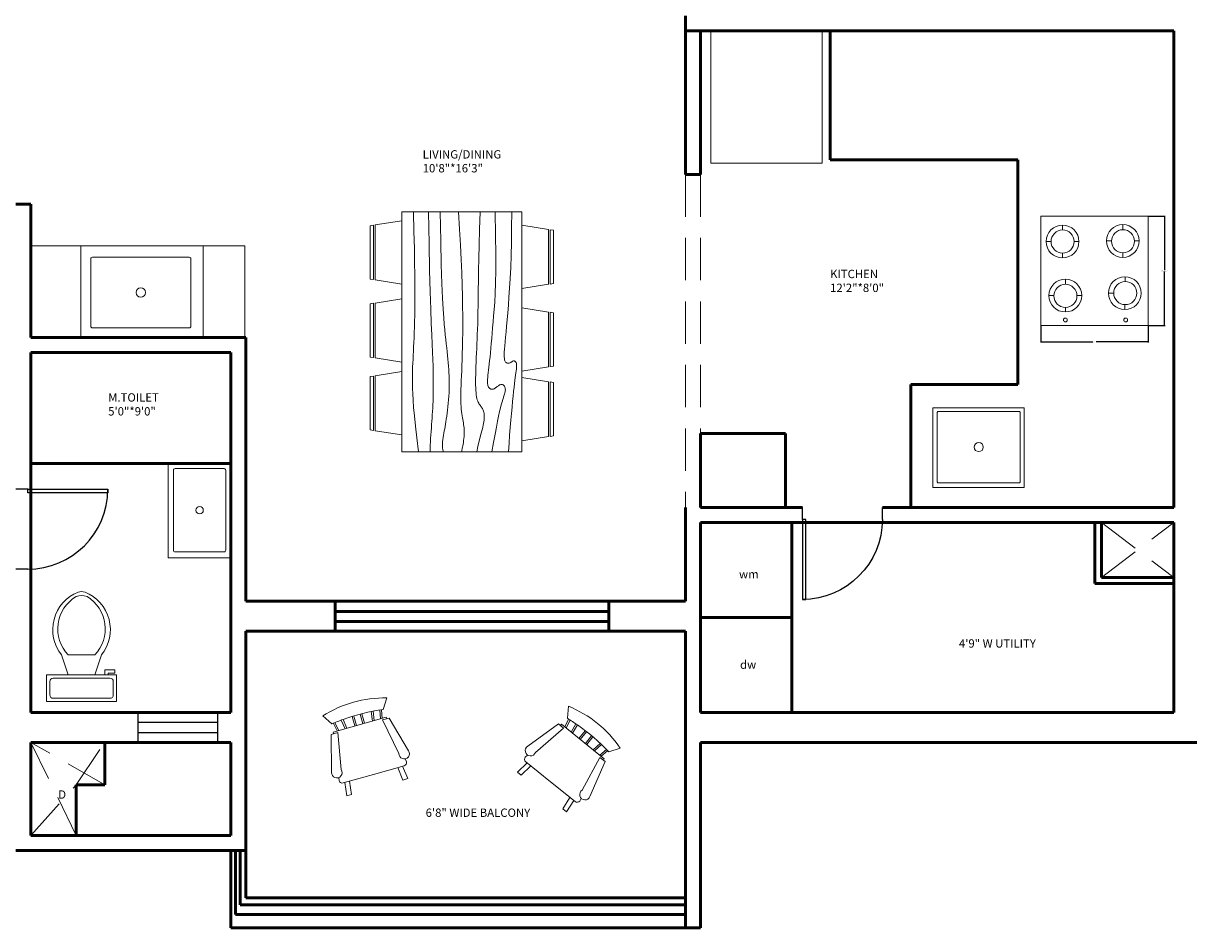
# Model space of a CAD drawing. Units: inches. Extents: x 291 to 2631, y 456 to 2623.
# Tile 2 of 22: x 550 to 900, y 456 to 728. Entities that reach past the tile are written whole.
import ezdxf

# ---------------------------------------------------------------- set-up
doc = ezdxf.new("R2010")
doc.units = ezdxf.units.IN
doc.linetypes.add('DASHED', pattern=[19.05, 12.7, -6.35])
for name, color, linetype, lineweight in [('A-ANNO-DIMS', 2, 'Continuous', 18), ('A-ANNO-TEXT', 3, 'Continuous', 25), ('A-AREA-IDEN', 7, 'Continuous', 25), ('A-DOOR', 3, 'Continuous', 25), ('A-EQPM', 8, 'Continuous', 18), ('A-FLOR-FIXT', 9, 'Continuous', 18), ('A-FLOR-OVHD', 1, 'DASHED', 18), ('A-FURN', 8, 'Continuous', 18), ('A-GLAZ', 4, 'Continuous', 25), ('A-WALL', 7, 'Continuous', 50)]:
    doc.layers.add(name, color=color, linetype=linetype, lineweight=lineweight)
doc.styles.get("Standard").update_dxf_attribs({"font": 'arial.ttf'})
doc.dimstyles.get("Standard").update_dxf_attribs({"dimtxt": 0.18, "dimasz": 0.18, "dimexe": 0.18, "dimexo": 0.0625, "dimgap": 0.09, "dimtad": 0, "dimtih": 1, "dimtoh": 1, "dimdec": 4, "dimzin": 0, "dimdsep": 46, "dimtxsty": 'Standard', "dimcen": 0.09, "dimadec": 0, "dimazin": 0, "dimtfac": 1, "dimtdec": 4, "dimtofl": 0, "dimtmove": 0, "dimatfit": 3, "dimfxl": 1, "dimtolj": 1, "dimtzin": 0, "dimarcsym": 0})

# ---------------------------------------------------------------- blocks, each defined once
blk = doc.blocks.new('*U2')
for p, q in [((0, 0), (0, -6)), ((40, 0), (40, -6))]:
    blk.add_line(p, q)
blk.add_lwpolyline([(0, 0), (0, 40), (1.75, 40), (1.75, 0)], close=True)
blk.add_arc((0, 0), 40, 0, 90)
blk = doc.blocks.new('Toilet - top')
for p, q in [((9.5, -6), (9.5, -2)), ((-10, -8.5), (-8, -8.5)), ((-10, -9.5), (-10, -8.5)), ((-7, -9.5), (-10, -9.5)), ((-8, -8.5), (-8, -8)), ((-7, -8), (-7, -9.5)), ((-4, -8), (-6, -14)), ((4, -8), (6, -14)), ((4, -14), (-4, -14))]:
    blk.add_line(p, q)
blk.add_lwpolyline([(10.5, -8), (10.5, 0), (-10.5, 0), (-10.5, -8)], close=True)
for points in [[(-9.5, -2), (-9.5, -6)], [(8.5, -1), (-8.5, -1)], [(-8.5, -7), (8.5, -7)]]:
    blk.add_lwpolyline(points)
for centre, radius, start, end in [((-8.62, -1.88), 0.884, 81.8699, 188.1301), ((8.62, -1.88), 0.884, 351.8699, 98.1301), ((-8.62, -6.12), 0.884, 171.8699, 278.1301), ((8.62, -6.12), 0.884, 261.8699, 8.1301), ((3.52, -21.58), 12.17, 141.4691, 247.9714), ((4.2, -21.82), 11.33, 136.3677, 238.9468), ((-3.52, -21.58), 12.17, 292.0284, 38.5307), ((-4.2, -21.82), 11.33, 301.053, 43.6321), ((0, -27.88), 4, 245.7318, 294.2682), ((0, -29), 4, 254.8605, 285.1395)]:
    blk.add_arc(centre, radius, start, end)
blk = doc.blocks.new('Chair - Rocking')
for p, q in [((-8, -4.5), (-10, -1.5)), ((8, -4.5), (10, -1.5)), ((-7.5, -4.5), (-7, -7)), ((-6.5, -7), (-7.02225, -4.43)), ((-4.5, -7), (-4.96674, -4.19951)), ((-4, -7), (-4.40532, -4.16272)), ((-1.5, -4.05012), (-1.5, -7)), ((-1, -7), (-1, -4.05012)), ((1, -7), (1, -4.04655)), ((1.5, -4.05012), (1.5, -7)), ((4, -7), (4.40187, -4.18694)), ((4.5, -7), (4.96761, -4.19437)), ((6.5, -7), (7, -4.4057)), ((7.5, -4.5), (7, -7)), ((-9, -7.5), (-12, -18.49999)), ((-7, -7.5), (-9, -7.5)), ((-9, -18.49999), (-7, -7.5)), ((-8.23428, -6.99939), (-8.3093, -7.47958)), ((-8.23041, -7), (8.23915, -7)), ((7, -7.5), (9, -7.5)), ((9, -18.49999), (7, -7.5)), ((8.31071, -7.48854), (8.23449, -7.00073)), ((9, -7.5), (12, -18.49999)), ((-10.36644, -20.64523), (-10.5, -21.49999)), ((10.5, -21.49999), (10.3575, -20.58798)), ((-9, -22.49999), (-9.5, -26.49999)), ((0, -22.49999), (-9.5, -22.49999)), ((-8, -26.49999), (-7.5, -22.49999)), ((0, -22.49999), (9.5, -22.49999)), ((8, -26.49999), (7.5, -22.49999)), ((9, -22.49999), (9.5, -26.49999)), ((-9.5, -26.49999), (-8, -26.49999)), ((9.5, -26.49999), (8, -26.49999))]:
    blk.add_line(p, q)
for centre, radius, start, end in [((0, -34.08333), 34.08333, 72.93847, 107.0615), ((0, -68.25004), 64.25, 93.92211, 97.15267), ((0, -68.25004), 64.25, 82.84733, 93.92211), ((-10.5, -18.99999), 1.58114, 161.5651, 18.43495), ((10.5, -18.99999), 1.58114, 161.5651, 18.43495), ((-9.5, -21.49999), 1, 180, 270), ((9.5, -21.49999), 1, 270, 0)]:
    blk.add_arc(centre, radius, start, end)
blk = doc.blocks.new('WIN-600')
for p, q in [((24, 9), (0, 9)), ((0, 9), (0, 0)), ((24, 0), (24, 9)), ((24, 6), (0, 6)), ((0, 3), (24, 3)), ((0, 0), (24, 0))]:
    blk.add_line(p, q)
blk = doc.blocks.new('COOKTOP-B')
for p, q in [((6.54, 28.68), (6.54, 30.14)), ((24.62, 30.31), (24.62, 28.76)), ((1.62, 25.22), (3.08, 25.22)), ((10, 25.22), (11.46, 25.22)), ((19.7, 25.39), (21.21, 25.39)), ((28.13, 25.39), (29.54, 25.39)), ((6.54, 21.76), (6.54, 20.3)), ((24.62, 21.83), (24.62, 20.47)), ((25.35, 14.65), (25.34, 13.21)), ((7.38, 13.92), (7.38, 12.38)), ((2.46, 9), (3.95, 9)), ((10.87, 9), (12.3, 9)), ((20.32, 9.73), (21.89, 9.73)), ((7.38, 5.46), (7.38, 4.08)), ((25.26, 6.28), (25.24, 4.81))]:
    blk.add_line(p, q)
blk.add_lwpolyline([(0, 32.79), (32.25, 32.79), (32.25, 0), (0, 0)], close=True)
for centre, radius in [((6.54, 25.22), 4.92), ((6.54, 25.22), 3.46), ((24.62, 25.39), 4.92), ((24.67, 25.29), 3.46), ((25.24, 9.73), 4.92), ((7.38, 9), 4.92), ((7.41, 8.92), 3.46), ((25.35, 9.74), 3.46), ((7.38, 1.69), 0.572), ((25.5, 1.69), 0.572)]:
    blk.add_circle(centre, radius)
blk = doc.blocks.new('*D50')
at = {"layer": 'A-ANNO-DIMS', "color": 0, "lineweight": -2, "transparency": 16777216}
for p, q in [((887.42, 669.83), (892.46, 669.83)), ((892.28, 669.65), (892.28, 653.62)), ((892.28, 637.22), (892.28, 653.25)), ((887.42, 637.04), (892.46, 637.04))]:
    blk.add_line(p, q, dxfattribs=at)
at = {"layer": 'A-ANNO-DIMS', "color": 0, "transparency": 16777216}
for points in [[(892.25, 669.65), (892.31, 669.65), (892.28, 669.83)], [(892.25, 637.22), (892.31, 637.22), (892.28, 637.04)]]:
    blk.add_solid(points, dxfattribs=at)
at = {"layer": 'DEFPOINTS', "color": 0, "transparency": 16777216}
for p in [(887.36, 669.83), (892.28, 669.83), (887.36, 637.04)]:
    blk.add_point(p, dxfattribs=at)
at = {"layer": 'A-ANNO-DIMS', "color": 0, "transparency": 16777216, "insert": (892.28, 653.44), "char_height": 0.18, "attachment_point": 5}
blk.add_mtext('\\A1;COOKTOP B 33 TYP.', dxfattribs=at)
blk = doc.blocks.new('*D51')
at = {"layer": 'A-ANNO-DIMS', "color": 0, "lineweight": -2, "transparency": 16777216}
for p, q in [((855.11, 636.98), (855.11, 631.94)), ((887.36, 636.98), (887.36, 631.94)), ((855.29, 632.12), (870.7, 632.12)), ((887.18, 632.12), (871.76, 632.12))]:
    blk.add_line(p, q, dxfattribs=at)
at = {"layer": 'A-ANNO-DIMS', "color": 0, "transparency": 16777216}
for points in [[(855.29, 632.15), (855.29, 632.09), (855.11, 632.12)], [(887.18, 632.15), (887.18, 632.09), (887.36, 632.12)]]:
    blk.add_solid(points, dxfattribs=at)
at = {"layer": 'DEFPOINTS', "color": 0, "transparency": 16777216}
for p in [(855.11, 637.04), (887.36, 637.04), (887.36, 632.12)]:
    blk.add_point(p, dxfattribs=at)
at = {"layer": 'A-ANNO-DIMS', "color": 0, "transparency": 16777216, "insert": (871.23, 632.12), "char_height": 0.18, "attachment_point": 5}
blk.add_mtext('\\A1;32 TYP.', dxfattribs=at)

msp = doc.modelspace()

# ---------------------------------------------------------------- linework, layer by layer
at = {"layer": 'A-FLOR-OVHD'}
for p, q in [((748.5, 682.38), (748.5, 582.48)), ((753, 682.38), (753, 604.64)), ((873.34, 577.98), (895, 561.42)), ((873.34, 561.42), (895, 577.98)), ((565.65, 484.08), (552, 511.98)), ((574.2, 499.28), (552, 511.98)), ((565.65, 499.28), (574.2, 511.98)), ((552, 484.08), (565.65, 499.28))]:
    msp.add_line(p, q, dxfattribs=at)
at = {"layer": 'A-FURN'}
for p, q in [((655.33, 667.22), (663.33, 668.47)), ((663.33, 671.18), (663.33, 599.18)), ((699.33, 671.18), (663.33, 671.18)), ((699.33, 599.18), (699.33, 671.18)), ((653.83, 666.99), (654.83, 667.15)), ((653.83, 666.99), (653.83, 650.99)), ((654.83, 650.83), (654.83, 667.14)), ((655.33, 667.22), (655.33, 650.75)), ((707.33, 665.89), (699.33, 667.14)), ((707.33, 665.88), (707.33, 649.41)), ((707.83, 649.49), (707.83, 665.81)), ((708.83, 665.65), (707.83, 665.81)), ((708.83, 665.65), (708.83, 649.65)), ((654.83, 650.83), (653.83, 650.99)), ((663.33, 649.51), (655.33, 650.76)), ((699.33, 648.17), (707.33, 649.42)), ((707.83, 649.5), (708.83, 649.65)), ((653.83, 643.58), (654.83, 643.73)), ((653.83, 643.58), (653.83, 627.58)), ((654.83, 627.42), (654.83, 643.73)), ((655.33, 643.81), (663.33, 645.06)), ((655.33, 643.81), (655.33, 627.34)), ((707.33, 641.11), (699.33, 642.36)), ((707.33, 641.1), (707.33, 624.63)), ((708.83, 640.87), (707.83, 641.03)), ((707.83, 624.71), (707.83, 641.03)), ((708.83, 640.87), (708.83, 624.87)), ((654.83, 627.42), (653.83, 627.58)), ((663.33, 626.09), (655.33, 627.34)), ((655.33, 621.96), (663.33, 623.22)), ((699.33, 623.39), (707.33, 624.64)), ((707.83, 624.72), (708.83, 624.87)), ((653.83, 621.73), (654.83, 621.89)), ((653.83, 621.73), (653.83, 605.73)), ((654.83, 605.57), (654.83, 621.88)), ((655.33, 621.96), (655.33, 605.49)), ((707.33, 620.2), (699.33, 621.45)), ((707.33, 620.2), (707.33, 603.73)), ((708.83, 619.97), (707.83, 620.13)), ((707.83, 603.81), (707.83, 620.12)), ((708.83, 619.97), (708.83, 603.97)), ((654.83, 605.57), (653.83, 605.73)), ((663.33, 604.25), (655.33, 605.5)), ((699.33, 602.48), (707.33, 603.74)), ((707.83, 603.81), (708.83, 603.97)), ((663.33, 599.18), (699.33, 599.18))]:
    msp.add_line(p, q, dxfattribs=at)
for points in [[(756.07, 725.48), (789.55, 725.48), (789.55, 685.78), (756.07, 685.78)], [(552, 633.48), (616.22, 633.48), (616.22, 660.97), (552, 660.97)], [(566.99, 660.97), (603.69, 660.97), (603.69, 633.48), (566.99, 633.48)], [(822.72, 612.37), (850.16, 612.37), (850.16, 588.47), (822.72, 588.47)], [(612, 595.7), (593.22, 595.7), (593.22, 567.32), (612, 567.32)]]:
    msp.add_lwpolyline(points, close=True, dxfattribs=at)
for points in [[(666.83, 671.18), (666.99, 665.26), (667.12, 660.21), (667.2, 655.91), (667.25, 652.25), (667.28, 649.15), (667.28, 646.48), (667.27, 644.15), (667.24, 642.05), (667.21, 640.1), (667.17, 638.27), (667.12, 636.55), (667.07, 634.93), (667.01, 633.41), (666.95, 631.98), (666.89, 630.63), (666.83, 629.34), (666.77, 628.12), (666.71, 626.94), (666.65, 625.78), (666.6, 624.63), (666.57, 623.46), (666.54, 622.25), (666.53, 620.98), (666.54, 619.63), (666.56, 618.18), (666.62, 616.56), (666.73, 614.7), (666.89, 612.51), (667.11, 609.95), (667.42, 606.91), (667.82, 603.35), (668.33, 599.18)], [(671.33, 671.18), (671.51, 661.58), (671.7, 653.64), (671.88, 647.16), (672.05, 641.92), (672.2, 637.7), (672.35, 634.3), (672.47, 631.5), (672.58, 629.09), (672.66, 626.9), (672.72, 624.87), (672.76, 623.01), (672.79, 621.28), (672.79, 619.69), (672.79, 618.22), (672.77, 616.86), (672.74, 615.59), (672.71, 614.41), (672.67, 613.31), (672.62, 612.26), (672.56, 611.25), (672.5, 610.27), (672.43, 609.3), (672.36, 608.33), (672.29, 607.34), (672.21, 606.33), (672.13, 605.29), (672.05, 604.25), (671.98, 603.2), (671.92, 602.16), (671.87, 601.13), (671.84, 600.14), (671.83, 599.18)], [(674.83, 671.18), (675.02, 662.36), (675.2, 655.26), (675.39, 649.65), (675.57, 645.29), (675.75, 641.95), (675.92, 639.41), (676.08, 637.44), (676.24, 635.8), (676.4, 634.31), (676.54, 632.9), (676.68, 631.59), (676.81, 630.35), (676.93, 629.17), (677.04, 628.05), (677.15, 626.97), (677.24, 625.93), (677.33, 624.91), (677.41, 623.9), (677.48, 622.91), (677.54, 621.93), (677.57, 620.94), (677.6, 619.95), (677.6, 618.95), (677.58, 617.93), (677.54, 616.89), (677.47, 615.83), (677.39, 614.78), (677.3, 613.73), (677.19, 612.7), (677.07, 611.7), (676.95, 610.75), (676.83, 609.84), (676.7, 609), (676.58, 608.21), (676.46, 607.46), (676.33, 606.75), (676.21, 606.08), (676.1, 605.42), (675.98, 604.77), (675.87, 604.13), (675.76, 603.49), (675.67, 602.85), (675.6, 602.21), (675.55, 601.58), (675.54, 600.95), (675.58, 600.34), (675.67, 599.75), (675.83, 599.18)], [(680.33, 671.18), (680.67, 665.97), (680.95, 661.2), (681.17, 656.83), (681.33, 652.83), (681.46, 649.18), (681.54, 645.83), (681.59, 642.76), (681.62, 639.93), (681.63, 637.31), (681.62, 634.89), (681.59, 632.64), (681.55, 630.56), (681.5, 628.62), (681.45, 626.81), (681.39, 625.11), (681.33, 623.51), (681.27, 621.99), (681.21, 620.54), (681.15, 619.18), (681.11, 617.89), (681.08, 616.69), (681.06, 615.58), (681.06, 614.54), (681.08, 613.59), (681.12, 612.73), (681.18, 611.94), (681.26, 611.22), (681.35, 610.56), (681.45, 609.95), (681.55, 609.39), (681.65, 608.85), (681.74, 608.34), (681.83, 607.85), (681.91, 607.37), (681.98, 606.89), (682.04, 606.41), (682.07, 605.92), (682.1, 605.41), (682.1, 604.89), (682.08, 604.34), (682.04, 603.77), (681.98, 603.18), (681.9, 602.59), (681.82, 602.01), (681.73, 601.48), (681.64, 600.99), (681.56, 600.56), (681.49, 600.22), (681.44, 599.97), (681.4, 599.79), (681.37, 599.67), (681.35, 599.59), (681.34, 599.52), (681.33, 599.44), (681.33, 599.33), (681.33, 599.18)], [(686.83, 671.18), (686.66, 665.89), (686.54, 661.25), (686.45, 657.17), (686.38, 653.6), (686.33, 650.48), (686.3, 647.73), (686.27, 645.29), (686.24, 643.09), (686.21, 641.09), (686.17, 639.23), (686.12, 637.52), (686.07, 635.92), (686.01, 634.4), (685.95, 632.96), (685.89, 631.55), (685.83, 630.18), (685.77, 628.8), (685.71, 627.44), (685.65, 626.1), (685.6, 624.8), (685.56, 623.55), (685.52, 622.35), (685.5, 621.22), (685.49, 620.18), (685.5, 619.22), (685.53, 618.36), (685.56, 617.58), (685.62, 616.87), (685.69, 616.25), (685.78, 615.69), (685.88, 615.19), (685.99, 614.76), (686.13, 614.38), (686.27, 614.05), (686.43, 613.75), (686.59, 613.49), (686.75, 613.25), (686.92, 613.03), (687.08, 612.81), (687.24, 612.59), (687.4, 612.37), (687.54, 612.14), (687.67, 611.89), (687.79, 611.62), (687.89, 611.34), (687.97, 611.03), (688.04, 610.7), (688.08, 610.34), (688.1, 609.95), (688.09, 609.53), (688.07, 609.09), (688.03, 608.62), (687.96, 608.14), (687.88, 607.64), (687.78, 607.12), (687.66, 606.59), (687.53, 606.05), (687.37, 605.47), (687.2, 604.81), (686.99, 604.04), (686.76, 603.13), (686.49, 602.03), (686.18, 600.73), (685.83, 599.18)], [(691.33, 671.18), (691.47, 664.15), (691.53, 658.35), (691.53, 653.6), (691.46, 649.74), (691.36, 646.62), (691.22, 644.05), (691.07, 641.89), (690.91, 639.97), (690.76, 638.15), (690.61, 636.4), (690.47, 634.73), (690.34, 633.15), (690.21, 631.65), (690.08, 630.24), (689.95, 628.91), (689.83, 627.68), (689.7, 626.54), (689.58, 625.48), (689.47, 624.52), (689.36, 623.65), (689.26, 622.85), (689.18, 622.13), (689.12, 621.49), (689.08, 620.93), (689.06, 620.43), (689.06, 620), (689.09, 619.62), (689.13, 619.3), (689.19, 619.03), (689.28, 618.79), (689.38, 618.6), (689.49, 618.43), (689.63, 618.28), (689.77, 618.16), (689.93, 618.07), (690.1, 618), (690.27, 617.96), (690.46, 617.95), (690.64, 617.96), (690.83, 618.01), (691.02, 618.09), (691.2, 618.19), (691.39, 618.31), (691.58, 618.45), (691.77, 618.59), (691.95, 618.74), (692.14, 618.88), (692.33, 619.01), (692.52, 619.13), (692.7, 619.22), (692.89, 619.3), (693.07, 619.35), (693.25, 619.38), (693.42, 619.37), (693.58, 619.33), (693.74, 619.26), (693.9, 619.15), (694.04, 619), (694.16, 618.82), (694.27, 618.6), (694.35, 618.36), (694.4, 618.1), (694.42, 617.81), (694.41, 617.51), (694.36, 617.19), (694.28, 616.83), (694.16, 616.44), (694.01, 615.98), (693.84, 615.46), (693.64, 614.84), (693.43, 614.13), (693.2, 613.3), (692.96, 612.34), (692.7, 611.22), (692.41, 609.9), (692.09, 608.35), (691.73, 606.53), (691.32, 604.42), (690.86, 601.98), (690.33, 599.18)], [(696.33, 671.18), (696.31, 666.35), (696.24, 661.98), (696.14, 658.03), (696.02, 654.45), (695.86, 651.21), (695.7, 648.27), (695.51, 645.59), (695.33, 643.13), (695.14, 640.87), (694.96, 638.78), (694.78, 636.87), (694.62, 635.14), (694.47, 633.58), (694.34, 632.2), (694.24, 630.98), (694.16, 629.93), (694.11, 629.04), (694.1, 628.3), (694.11, 627.69), (694.14, 627.2), (694.2, 626.81), (694.28, 626.5), (694.38, 626.27), (694.49, 626.09), (694.63, 625.96), (694.77, 625.85), (694.93, 625.79), (695.09, 625.75), (695.25, 625.74), (695.42, 625.75), (695.58, 625.79), (695.74, 625.84), (695.9, 625.91), (696.04, 625.99), (696.18, 626.08), (696.32, 626.17), (696.45, 626.25), (696.58, 626.32), (696.7, 626.38), (696.83, 626.43), (696.95, 626.45), (697.08, 626.44), (697.19, 626.41), (697.31, 626.36), (697.41, 626.29), (697.51, 626.19), (697.59, 626.07), (697.66, 625.93), (697.72, 625.76), (697.75, 625.56), (697.78, 625.33), (697.79, 625.05), (697.78, 624.73), (697.75, 624.36), (697.72, 623.92), (697.66, 623.43), (697.59, 622.86), (697.51, 622.21), (697.41, 621.46), (697.3, 620.61), (697.17, 619.64), (697.04, 618.53), (696.9, 617.29), (696.74, 615.88), (696.58, 614.32), (696.42, 612.59), (696.25, 610.7), (696.07, 608.67), (695.89, 606.5), (695.7, 604.18), (695.52, 601.74), (695.33, 599.18)]]:
    msp.add_lwpolyline(points, dxfattribs=at)
for points in [[(570.48, 657.54), (599.53, 657.54, -0.414214), (600.03, 657.04), (600.03, 636.87, -0.414214), (599.53, 636.37), (570.48, 636.37, -0.414214), (569.98, 636.87), (569.98, 657.04, -0.414214)], [(824.36, 611.26), (848.66, 611.26, -0.414214), (848.96, 610.96), (848.96, 590.18, -0.414214), (848.66, 589.88), (824.36, 589.88, -0.414214), (824.06, 590.18), (824.06, 610.96, -0.414214)], [(595.33, 594.13), (610.01, 594.13, -0.414214), (610.51, 593.63), (610.51, 569.66, -0.414214), (610.01, 569.16), (595.33, 569.16, -0.414214), (594.83, 569.66), (594.83, 593.63, -0.414214)]]:
    msp.add_lwpolyline(points, format="xyb", close=True, dxfattribs=at)
for centre, radius in [((585.01, 646.96), 1.43), ((836.51, 600.57), 1.36), ((602.67, 581.64), 1.11)]:
    msp.add_circle(centre, radius, dxfattribs=at)
at = {"layer": 'A-WALL'}
for p, q in [((748.5, 729.98), (748.5, 682.38)), ((895, 725.48), (748.5, 725.48)), ((753, 725.48), (753, 682.38)), ((791.92, 686.75), (791.92, 725.48)), ((895, 725.48), (895, 582.48)), ((848.18, 686.75), (791.92, 686.75)), ((848.18, 619.39), (848.18, 686.75)), ((748.5, 682.38), (753, 682.38)), ((552, 673.48), (547.5, 673.48)), ((552, 673.48), (552, 633.48)), ((616.5, 633.48), (552, 633.48)), ((616.5, 633.48), (616.5, 554.39)), ((612, 628.98), (552, 628.98)), ((552, 628.98), (552, 520.98)), ((612, 628.98), (612, 520.98)), ((816.13, 582.48), (816.13, 619.39)), ((816.13, 619.39), (848.18, 619.39)), ((753, 604.64), (778.52, 604.64)), ((753, 604.64), (753, 582.48)), ((778.52, 604.64), (778.52, 582.48)), ((552, 595.7), (612, 595.7)), ((748.5, 582.48), (748.5, 554.39)), ((783.56, 582.48), (753, 582.48)), ((895, 582.48), (807.56, 582.48)), ((895, 577.98), (753, 577.98)), ((753, 577.98), (753, 520.98)), ((780.41, 577.98), (780.41, 520.98)), ((871.38, 577.98), (871.38, 559.68)), ((873.34, 577.98), (873.34, 561.42)), ((895, 577.98), (895, 520.98)), ((871.38, 559.68), (895, 559.68)), ((873.34, 561.42), (895, 561.42)), ((616.5, 554.39), (748.5, 554.39)), ((643.35, 554.39), (643.35, 545.39)), ((725.5, 554.39), (725.5, 545.39)), ((643.35, 551.21), (725.5, 551.21)), ((780.41, 549.48), (753, 549.48)), ((643.35, 548.25), (725.5, 548.25)), ((616.5, 545.39), (748.5, 545.39)), ((616.5, 545.39), (616.5, 511.98)), ((748.5, 545.39), (748.5, 511.98)), ((612, 520.98), (552, 520.98)), ((895, 520.98), (753, 520.98)), ((612, 511.98), (552, 511.98)), ((552, 511.98), (552, 484.08)), ((574.2, 499.28), (574.2, 511.98)), ((612, 511.98), (612, 484.08)), ((616.5, 511.98), (616.5, 465.39)), ((748.5, 511.98), (748.5, 456.39)), ((904, 511.98), (753, 511.98)), ((753, 511.98), (753, 456.39)), ((565.65, 484.08), (565.65, 499.28)), ((565.65, 499.28), (574.2, 499.28)), ((552, 484.08), (612, 484.08)), ((547.5, 479.56), (616.5, 479.56)), ((612, 479.56), (612, 456.39)), ((613.4, 479.56), (613.4, 460.38)), ((614.81, 479.5), (614.81, 463.28)), ((616.5, 465.39), (748.5, 465.39)), ((614.81, 463.28), (748.5, 463.28)), ((613.4, 460.38), (748.5, 460.38)), ((612, 456.39), (616.5, 456.39)), ((616.5, 456.39), (748.5, 456.39)), ((753, 456.39), (748.5, 456.39))]:
    msp.add_line(p, q, dxfattribs=at)

# ---------------------------------------------------------------- block references
at = {"layer": 'A-DOOR', "yscale": 0.6, "zscale": 0.6}
for p, xscale, rotation in [((551.1, 587.94), 0.6, 270), ((783.56, 578.88), -0.6, 180)]:
    msp.add_blockref('*U2', p, dxfattribs=dict(at, xscale=xscale, rotation=rotation))
at = {"layer": 'A-EQPM'}
msp.add_blockref('COOKTOP-B', (855.11, 637.04), dxfattribs=at)
at = {"layer": 'A-FLOR-FIXT', "rotation": 180}
msp.add_blockref('Toilet - top', (567.23, 524.21), dxfattribs=at)
at = {"layer": 'A-FURN'}
for p, rotation in [((648.82, 524.05), 15.67595765379025), ((722.08, 517.7), 321.0741999402937)]:
    msp.add_blockref('Chair - Rocking', p, dxfattribs=dict(at, rotation=rotation))
at = {"layer": 'A-GLAZ', "rotation": 180}
msp.add_blockref('WIN-600', (608.1, 520.98), dxfattribs=at)

# ---------------------------------------------------------------- texts
at = {"layer": 'A-ANNO-TEXT', "char_height": 2.5, "attachment_point": 1}
for s, width, insert in [('wm', 14.1058, (764.55, 563.7)), ('dw', 14.5729, (764.86, 536.56)), ('D', 1.6709, (560.24, 497.6))]:
    msp.add_mtext_dynamic_manual_height_columns(s, width=width, gutter_width=12.5, heights=[0], dxfattribs=dict(at, insert=insert))
at = {"layer": 'A-AREA-IDEN', "char_height": 2.5, "attachment_point": 1}
for s, width, insert in [('LIVING/DINING\\P10\'8"*16\'3"', 69.7388, (669.61, 689.66)), ('KITCHEN\\P12\'2"*8\'0"', 65.5453, (791.88, 653.78)), ('M.TOILET\\P5\'0"*9\'0"', 47.4151, (575.23, 616.73)), ('4\'9" W UTILITY', 80.448, (830.55, 542.92)), ('6\'8" WIDE BALCONY', 84.4828, (670.51, 492.14))]:
    msp.add_mtext_dynamic_manual_height_columns(s, width=width, gutter_width=12.5, heights=[0], dxfattribs=dict(at, insert=insert))

# ---------------------------------------------------------------- dimensions: what is measured, and where the dimension line sits
at = {"layer": 'A-ANNO-DIMS'}
dim = msp.add_linear_dim(base=(892.28, 669.83), p1=(887.36, 637.04), p2=(887.36, 669.83), angle=90, text='COOKTOP B <> TYP.', dimstyle='Standard', override={"dimdec": 0, "dimlfac": 1, "dimrnd": 0, "dimzin": 0, "dimdsep": 46, "dimlunit": 2}, dxfattribs=at)
dim.commit()
dim.dimension.update_dxf_attribs({"geometry": '*D50', "text_midpoint": (892.28, 653.44)})
dim = msp.add_linear_dim(base=(887.36, 632.12), p1=(855.11, 637.04), p2=(887.36, 637.04), text='<> TYP.', dimstyle='Standard', override={"dimdec": 0, "dimlfac": 1, "dimrnd": 0, "dimzin": 0, "dimdsep": 46, "dimlunit": 2}, dxfattribs=at)
dim.commit()
dim.dimension.update_dxf_attribs({"geometry": '*D51', "text_midpoint": (871.23, 632.12)})

doc.saveas('drawing.dxf')
